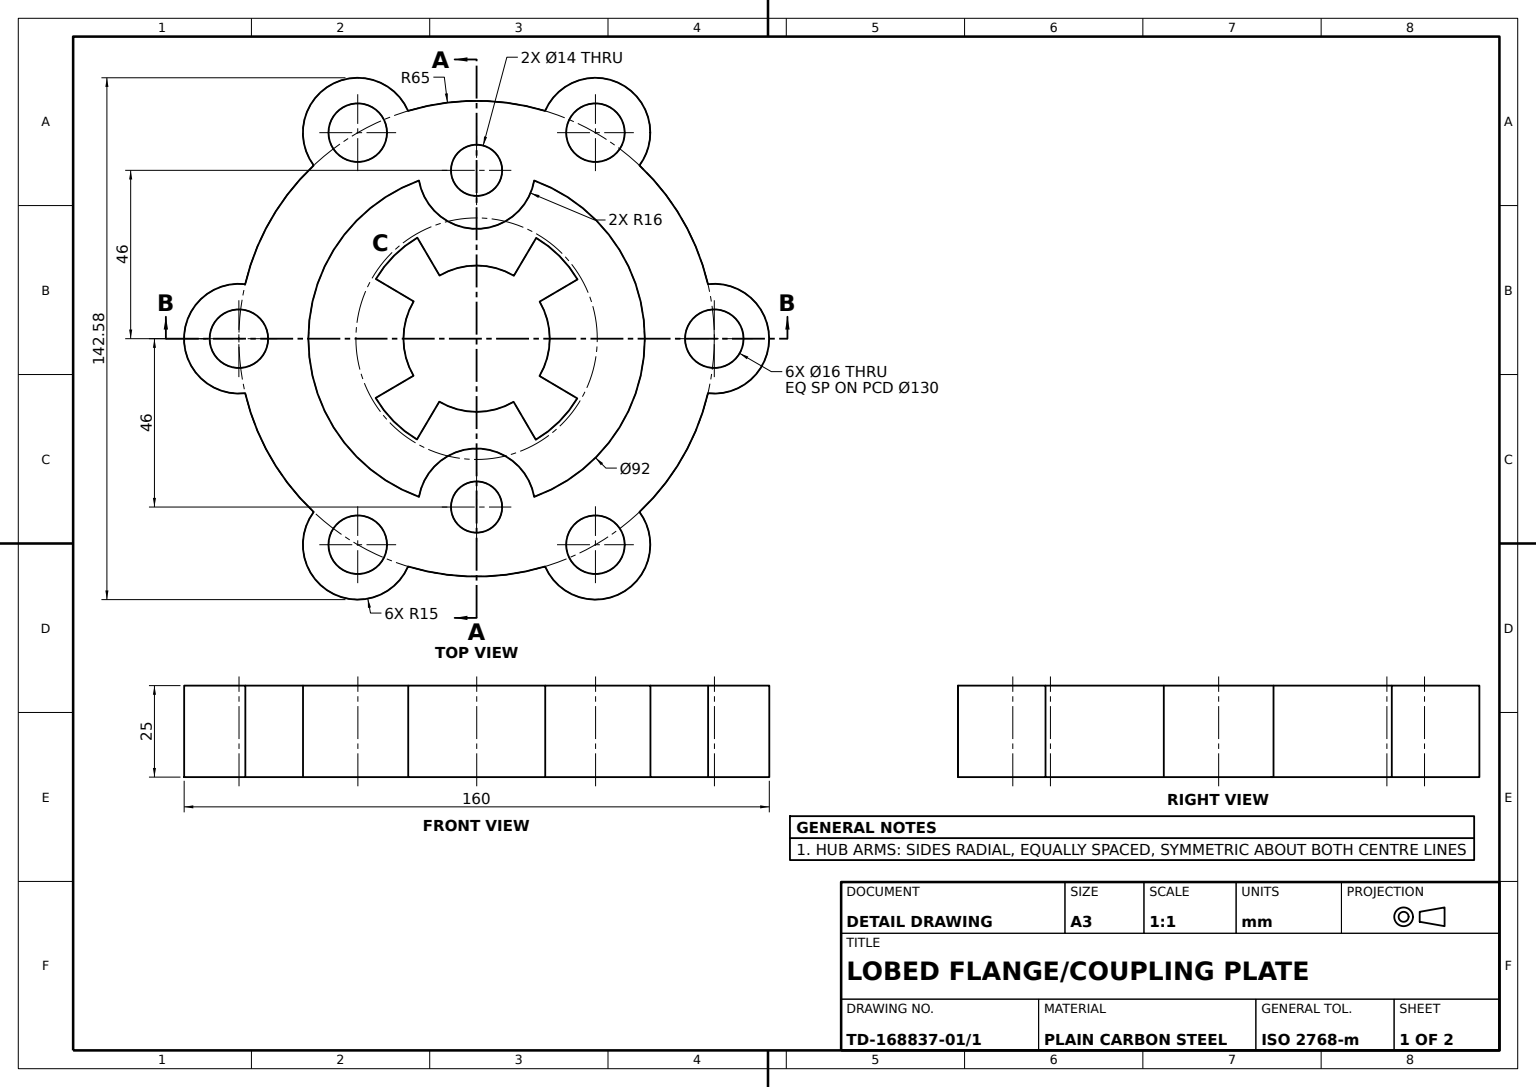
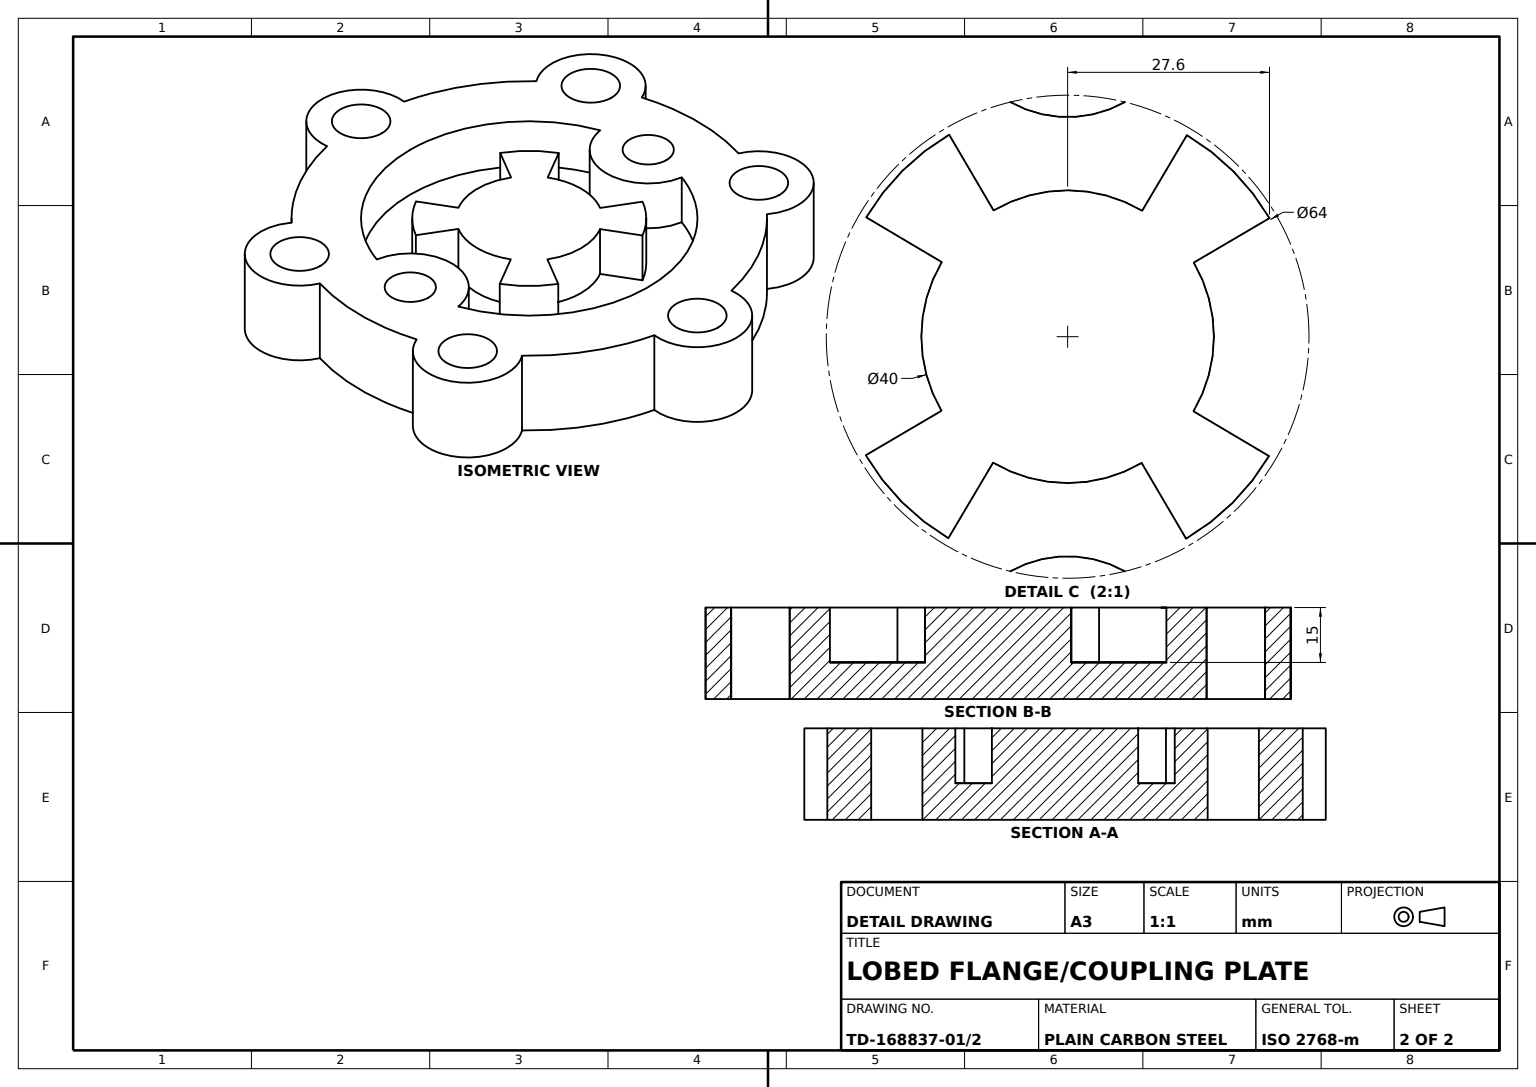
from build123d import *

# Parameters (mm, degrees)
FLANGE_PLATE_DEPTH        = 25
BOLT_HOLES_SKETCH_R       = 8
BOLT_HOLES_6X_16_DEPTH    = 25
ANNULAR_RECESS_92_DEPTH   = 15
LUG_HOLES_SKETCH_R        = 7
LUG_HOLES_2X_14_DEPTH     = 111.034083526
KEYED_CENTRE_HUB_40_DEPTH = 15


with BuildPart() as part:
    # Flange Profile Sketch → Flange Plate (new body)
    with BuildSketch(Plane(origin=(0, 0, 0), x_dir=(1, 0, 0), z_dir=(0, 1, 0))):
        with BuildLine():
            ThreePointArc((-14.89981335, 63.269230769), (-32.5, 56.291651246), (-47.342854449, 44.538232258))
            ThreePointArc((-47.342854449, 44.538232258), (-69.282032303, 40), (-62.242667799, 18.730998512))
            ThreePointArc((-62.242667799, 18.730998512), (-65, 0), (-62.242667799, -18.730998512))
            ThreePointArc((-62.242667799, -18.730998512), (-69.282032303, -40), (-47.342854449, -44.538232258))
            ThreePointArc((-47.342854449, -44.538232258), (-32.5, -56.291651246), (-14.89981335, -63.269230769))
            ThreePointArc((-14.89981335, -63.269230769), (0, -80), (14.89981335, -63.269230769))
            ThreePointArc((14.89981335, -63.269230769), (32.5, -56.291651246), (47.342854449, -44.538232258))
            ThreePointArc((47.342854449, -44.538232258), (69.282032303, -40), (62.242667799, -18.730998512))
            ThreePointArc((62.242667799, -18.730998512), (65, 0), (62.242667799, 18.730998512))
            ThreePointArc((62.242667799, 18.730998512), (69.282032303, 40), (47.342854449, 44.538232258))
            ThreePointArc((47.342854449, 44.538232258), (32.5, 56.291651246), (14.89981335, 63.269230769))
            ThreePointArc((14.89981335, 63.269230769), (0, 80), (-14.89981335, 63.269230769))
        make_face()
    extrude(amount=FLANGE_PLATE_DEPTH)

    # Bolt Holes Sketch → Bolt Holes 6xØ16 (cut)
    with BuildSketch(Plane(origin=(0, 25, 0), x_dir=(1, 0, 0), z_dir=(0, 1, 0))):
        with Locations(Location((0, 65, 0), (0, 0, 270))):
            Circle(BOLT_HOLES_SKETCH_R)
        with Locations(Location((56.291651246, 32.5, 0), (0, 0, 270))):
            Circle(BOLT_HOLES_SKETCH_R)
        with Locations(Location((56.291651246, -32.5, 0), (0, 0, 270))):
            Circle(BOLT_HOLES_SKETCH_R)
        with Locations(Location((0, -65, 0), (0, 0, 270))):
            Circle(BOLT_HOLES_SKETCH_R)
        with Locations(Location((-56.291651246, -32.5, 0), (0, 0, 270))):
            Circle(BOLT_HOLES_SKETCH_R)
        with Locations(Location((-56.291651246, 32.5, 0), (0, 0, 270))):
            Circle(BOLT_HOLES_SKETCH_R)
    extrude(amount=-BOLT_HOLES_6X_16_DEPTH, mode=Mode.SUBTRACT)

    # Recess Sketch → Annular Recess Ø92 (cut)
    with BuildSketch(Plane(origin=(0, 25, 0), x_dir=(1, 0, 0), z_dir=(0, 1, 0))):
        with BuildLine():
            ThreePointArc((-43.217391304, -15.756176213), (0, -46), (43.217391304, -15.756176213))
            ThreePointArc((43.217391304, -15.756176213), (30, 0), (43.217391304, 15.756176213))
            ThreePointArc((43.217391304, 15.756176213), (0, 46), (-43.217391304, 15.756176213))
            ThreePointArc((-43.217391304, 15.756176213), (-30, 0), (-43.217391304, -15.756176213))
        make_face()
    extrude(amount=-ANNULAR_RECESS_92_DEPTH, mode=Mode.SUBTRACT)

    # Lug Holes Sketch → Lug Holes 2xØ14 (cut, through all)
    with BuildSketch(Plane(origin=(0, 25, 0), x_dir=(1, 0, 0), z_dir=(0, 1, 0))):
        with Locations(Location((-46, 0, 0), (0, 0, 270))):
            Circle(LUG_HOLES_SKETCH_R)
        with Locations(Location((46, 0, 0), (0, 0, 270))):
            Circle(LUG_HOLES_SKETCH_R)
    extrude(amount=-LUG_HOLES_2X_14_DEPTH, mode=Mode.SUBTRACT)

    # Centre Hub Sketch → Keyed Centre Hub Ø40 (add)
    with BuildSketch(Plane(origin=(0, 10, 0), x_dir=(1, 0, 0), z_dir=(0, 1, 0))):
        with BuildLine():
            Line((17.207997686, -10.192390085), (27.532796297, -16.307824137))
            ThreePointArc((27.532796297, -16.307824137), (22.581559349, -22.673181898), (16.196205348, -27.598603811))
            Line((16.196205348, -27.598603811), (10.122628343, -17.249127382))
            ThreePointArc((10.122628343, -17.249127382), (-0.040491828, -19.99995901), (-10.192390085, -17.207997686))
            Line((-10.192390085, -17.207997686), (-16.307824137, -27.532796297))
            ThreePointArc((-16.307824137, -27.532796297), (-22.673181898, -22.581559349), (-27.598603811, -16.196205348))
            Line((-27.598603811, -16.196205348), (-17.249127382, -10.122628343))
            ThreePointArc((-17.249127382, -10.122628343), (-19.99995901, 0.040491828), (-17.207997686, 10.192390085))
            Line((-17.207997686, 10.192390085), (-27.532796297, 16.307824137))
            ThreePointArc((-27.532796297, 16.307824137), (-22.581559349, 22.673181898), (-16.196205348, 27.598603811))
            Line((-16.196205348, 27.598603811), (-10.122628343, 17.249127382))
            ThreePointArc((-10.122628343, 17.249127382), (0.040491828, 19.99995901), (10.192390085, 17.207997686))
            Line((10.192390085, 17.207997686), (16.307824137, 27.532796297))
            ThreePointArc((16.307824137, 27.532796297), (22.673181898, 22.581559349), (27.598603811, 16.196205348))
            Line((27.598603811, 16.196205348), (17.249127382, 10.122628343))
            ThreePointArc((17.249127382, 10.122628343), (19.99995901, -0.040491828), (17.207997686, -10.192390085))
        make_face()
    extrude(amount=KEYED_CENTRE_HUB_40_DEPTH)


solid = part.part
